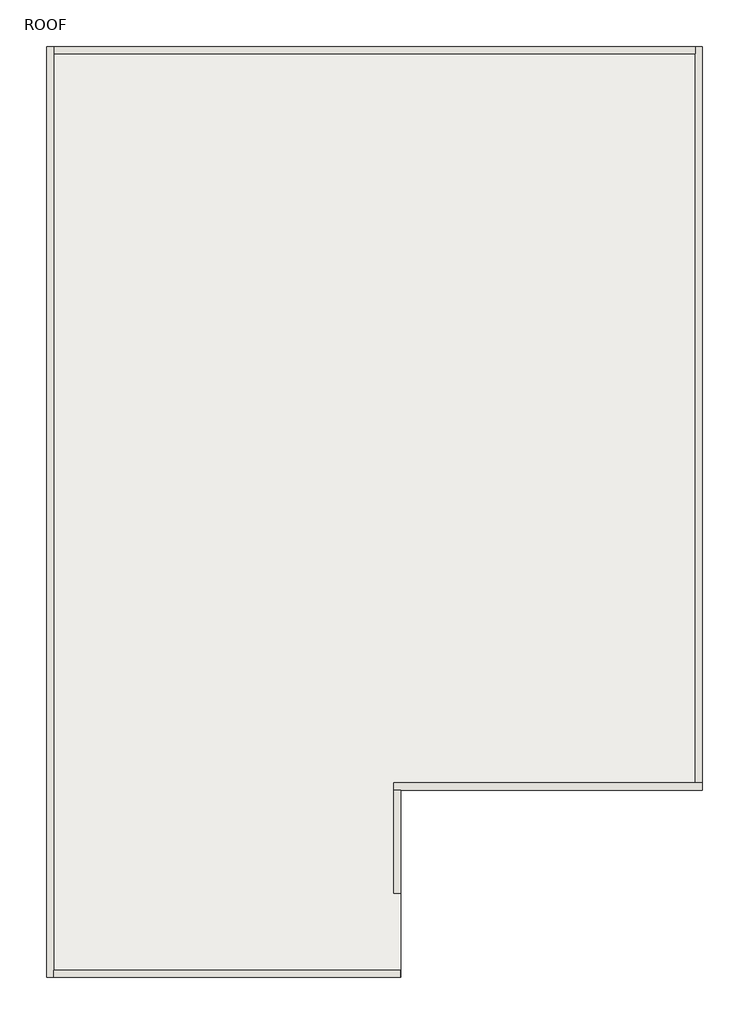
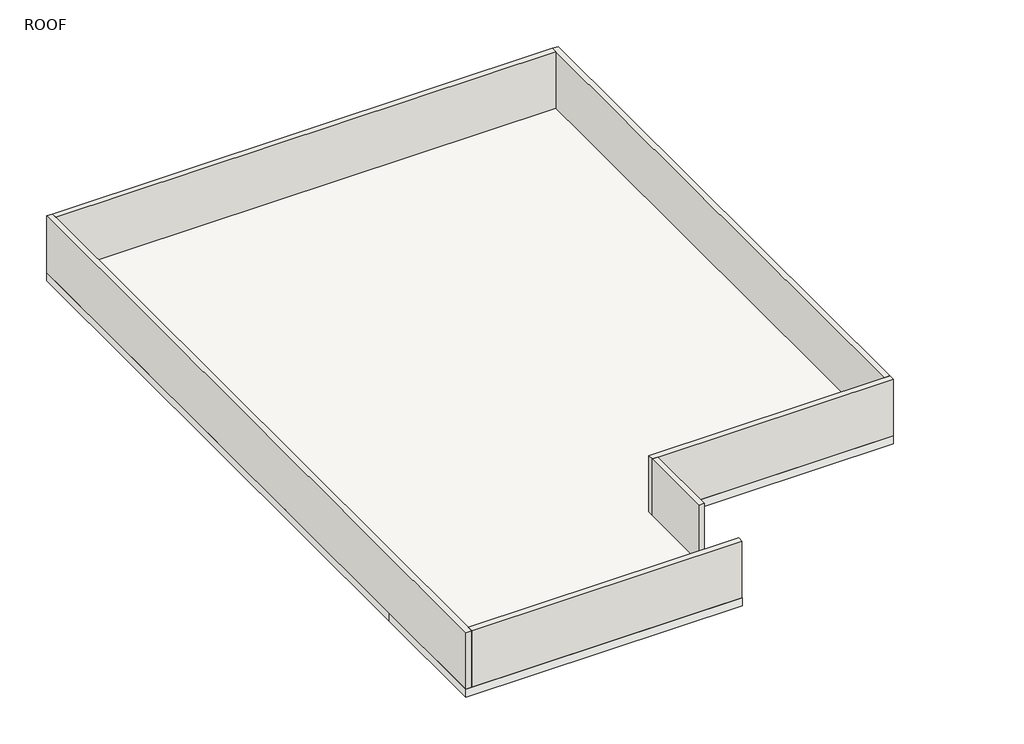
# One storey: 6 walls, 1 slab.
"""IFC4 building model written with IfcOpenShell, lengths in millimetres."""

from ifc_helpers import new_model, si_unit, frame, origin, place, context, project, spatial, polyline, outline, extrude, faceted_brep, element, save

model = new_model("IFC4")

# Units and contexts
model_context = context("Model", 3, world=origin())
ifc_project = project(units=[si_unit("LENGTHUNIT", "METRE", prefix="MILLI")], contexts=[model_context])

# Site, building, storey
site = spatial("IfcSite", under=ifc_project)
building = spatial("IfcBuilding", under=site)
storey = spatial("IfcBuildingStorey", under=building, Name="ROOF", Elevation=9601.2)

# Slab
placement = place(None, origin())
element("IfcSlab", 1, ObjectType="6\" floor", at=placement, inside=storey, context=model_context, shape_type="SweptSolid", body=[
    extrude(outline(polyline([(4406.9455952, 5921.9351347), (4406.9455952, -4415.8648653), (215.9455952, -4415.8648653), (215.9455952, -7021.8741001), (-4711.6544048, -7021.8741001), (-4711.6544048, -4637.8294487), (-4711.6544048, 5921.9351347), (4406.9455952, 5921.9351347)])), frame((0.0, 0.0, 9448.8), z_axis=(0.0, 0.0, 1.0), x_axis=(1.0, 0.0, 0.0)), (0.0, 0.0, 1.0), 152.4),
])

# Walls
element("IfcWall", 2, ObjectType="4\" wall", at=placement, inside=storey, context=model_context, shape_type="Brep", body=[
    faceted_brep([(-4711.6544048, 5921.9351347, 9601.2), (-4711.6544048, -7021.8741001, 9601.2), (-4711.6544048, -7021.8741001, 10668.0), (-4711.6544048, 5921.9351347, 10668.0), (-4610.0544048, 5921.9351347, 9601.2), (-4610.0544048, 5921.9351347, 10668.0), (-4610.0544048, 5820.3351347, 10668.0), (-4610.0544048, -6920.2741001, 10668.0), (-4610.0544048, -7021.8741001, 10668.0), (-4610.0544048, -7021.8741001, 9601.2), (-4610.0544048, -6920.2741001, 9601.2), (-4610.0544048, 5820.3351347, 9601.2)], [[[0, 1, 2, 3]], [[4, 5, 6, 7, 8, 9, 10, 11]], [[1, 0, 4, 11, 10, 9]], [[3, 2, 8, 7, 6, 5]], [[2, 1, 9, 8]], [[0, 3, 5, 4]]]),
])
element("IfcWall", 3, ObjectType="4\" wall", at=placement, inside=storey, context=model_context, shape_type="SweptSolid", body=[
    extrude(outline(polyline([(208.3455952, -7021.8741001), (-4610.0544048, -7021.8741001), (-4610.0544048, -6920.2741001), (208.3455952, -6920.2741001), (208.3455952, -7021.8741001)])), frame((0.0, 0.0, 9601.2), z_axis=(0.0, 0.0, 1.0), x_axis=(1.0, 0.0, 0.0)), (0.0, 0.0, 1.0), 1066.8),
])
element("IfcWall", 4, ObjectType="4\" wall", at=placement, inside=storey, context=model_context, shape_type="Brep", body=[
    faceted_brep([(114.3455952, -4415.8648653, 9601.2), (215.9455952, -4415.8648653, 9601.2), (4406.9455952, -4415.8648653, 9601.2), (4406.9455952, -4415.8648653, 10668.0), (215.9455952, -4415.8648653, 10668.0), (114.3455952, -4415.8648653, 10668.0), (114.3455952, -4314.2648653, 9601.2), (114.3455952, -4314.2648653, 10668.0), (4305.3455952, -4314.2648653, 10668.0), (4406.9455952, -4314.2648653, 10668.0), (4406.9455952, -4314.2648653, 9601.2), (4305.3455952, -4314.2648653, 9601.2)], [[[0, 1, 2, 3, 4, 5]], [[6, 7, 8, 9, 10, 11]], [[2, 1, 0, 6, 11, 10]], [[5, 4, 3, 9, 8, 7]], [[3, 2, 10, 9]], [[0, 5, 7, 6]]]),
])
element("IfcWall", 5, ObjectType="4\" wall", at=placement, inside=storey, context=model_context, shape_type="Brep", body=[
    faceted_brep([(4406.9455952, -4314.2648653, 9601.2), (4406.9455952, 5921.9351347, 9601.2), (4406.9455952, 5921.9351347, 10668.0), (4406.9455952, -4314.2648653, 10668.0), (4305.3455952, -4314.2648653, 9601.2), (4305.3455952, -4314.2648653, 10668.0), (4305.3455952, 5820.3351347, 10668.0), (4305.3455952, 5921.9351347, 10668.0), (4305.3455952, 5921.9351347, 9601.2), (4305.3455952, 5820.3351347, 9601.2)], [[[0, 1, 2, 3]], [[4, 5, 6, 7, 8, 9]], [[1, 0, 4, 9, 8]], [[3, 2, 7, 6, 5]], [[0, 3, 5, 4]], [[2, 1, 8, 7]]]),
])
element("IfcWall", 6, ObjectType="4\" wall", at=placement, inside=storey, context=model_context, shape_type="SweptSolid", body=[
    extrude(outline(polyline([(-4610.0544048, 5921.9351347), (4305.3455952, 5921.9351347), (4305.3455952, 5820.3351347), (-4610.0544048, 5820.3351347), (-4610.0544048, 5921.9351347)])), frame((0.0, 0.0, 9601.2), z_axis=(0.0, 0.0, 1.0), x_axis=(1.0, 0.0, 0.0)), (0.0, 0.0, 1.0), 1066.8),
])
element("IfcWall", 7, ObjectType="4\" wall", at=placement, inside=storey, context=model_context, shape_type="SweptSolid", body=[
    extrude(outline(polyline([(114.3455952, -5852.2556304), (114.3455952, -4415.8648653), (215.9455952, -4415.8648653), (215.9455952, -5852.2556304), (114.3455952, -5852.2556304)])), frame((0.0, 0.0, 9601.2), z_axis=(0.0, 0.0, 1.0), x_axis=(1.0, 0.0, 0.0)), (0.0, 0.0, 1.0), 1066.8),
])

save(model, "model.ifc")

# Revit data of these elements
# Type "6\" floor"
#   Function = 0
#   Layers, outside or top first: 0.5 ft no material (function 1)
# Type "4\" wall"
#   Layers, outside or top first: 0.333333 ft no material (function 1)
# Element 1 (IfcSlab, "6\" floor")
#   Height Offset From Level = 0.0 ft
#   Phase Created = New Construction
#   Materials on its faces: "Default Floor"
# Elements 2, 3, 4, 5, 6, 7 (IfcWall, "4\" wall")
#   Top Offset = 0.0 ft
#   Base Offset = 0.0 ft
#   Unconnected Height = 3.5 ft
#   wall height = 3.5 ft
#   Phase Created = New Construction
#   Base Constraint = ROOF
#   Materials on its faces: "Default Wall"
# Materials
#   "Default Floor": colour RGB 127 127 127, transparency 0, Cost = 0
#   "Default Wall": colour RGB 128 128 128, transparency 0, Cost = 0
